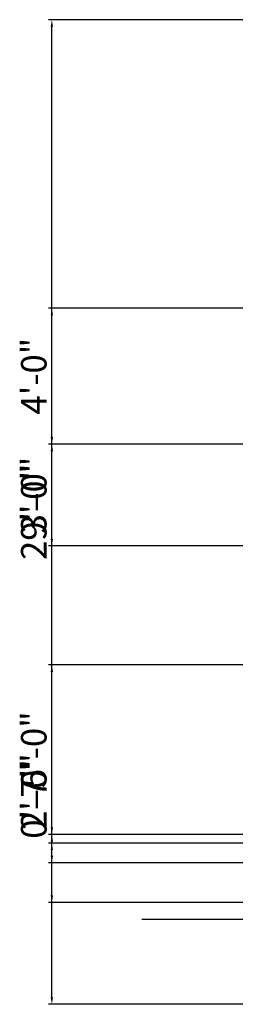
# Model space of a CAD drawing. Units: inches. Extents: x 600 to 1805, y 898 to 2057.
# Tile 1 of 5: x 1096 to 1172, y 938 to 1286. Entities that reach past the tile are written whole.
import ezdxf

# ---------------------------------------------------------------- set-up
doc = ezdxf.new("R2010")
doc.units = ezdxf.units.IN
doc.layers.add('A-ANNO-DIMS', color=2, linetype='Continuous', lineweight=18)
doc.layers.add('C-SITE', color=7, linetype='Continuous', lineweight=25)
doc.styles.get("Standard").update_dxf_attribs({"font": 'arial.ttf'})
doc.dimstyles.new('ISO-25', dxfattribs={"dimtxt": 9, "dimasz": 2.5, "dimexe": 1.25, "dimexo": 0.625, "dimtad": 1, "dimlunit": 3, "dimtxsty": 'Standard', "dimcen": 2.5, "dimadec": 0, "dimazin": 0, "dimtfac": 1, "dimtmove": 0, "dimatfit": 3, "dimfxl": 1, "dimarcsym": 0})

# ---------------------------------------------------------------- blocks, each defined once
blk = doc.blocks.new('*D42')
at = {"layer": 'A-ANNO-DIMS', "color": 0, "lineweight": -2, "transparency": 16777216}
for p, q in [((1406.71, 1285.8), (1106.33, 1285.8)), ((1107.58, 940.3), (1107.58, 1283.3)), ((1183.78, 937.8), (1106.33, 937.8))]:
    blk.add_line(p, q, dxfattribs=at)
at = {"layer": 'A-ANNO-DIMS', "color": 0, "transparency": 16777216}
for points in [[(1107.16, 1283.3), (1107.99, 1283.3), (1107.58, 1285.8)], [(1107.16, 940.3), (1107.99, 940.3), (1107.58, 937.8)]]:
    blk.add_solid(points, dxfattribs=at)
at = {"layer": 'Defpoints', "color": 0, "transparency": 16777216}
for p in [(1107.58, 1285.8), (1407.34, 1285.8), (1184.4, 937.8)]:
    blk.add_point(p, dxfattribs=at)
at = {"layer": 'A-ANNO-DIMS', "color": 0, "transparency": 16777216, "insert": (1102.36, 1111.8), "char_height": 9, "attachment_point": 5, "rotation": 90}
blk.add_mtext('29\'-0"', dxfattribs=at)
blk = doc.blocks.new('*D47')
at = {"layer": 'A-ANNO-DIMS', "color": 0, "lineweight": -2, "transparency": 16777216}
for p, q in [((1107.58, 994.8), (1107.58, 1022.48)), ((1562.71, 994.8), (1106.33, 994.8)), ((1107.58, 990.3), (1107.58, 992.3)), ((1562.71, 987.8), (1106.33, 987.8))]:
    blk.add_line(p, q, dxfattribs=at)
at = {"layer": 'A-ANNO-DIMS', "color": 0, "transparency": 16777216}
for points in [[(1107.16, 992.3), (1107.99, 992.3), (1107.58, 994.8)], [(1107.16, 990.3), (1107.99, 990.3), (1107.58, 987.8)]]:
    blk.add_solid(points, dxfattribs=at)
at = {"layer": 'Defpoints', "color": 0, "transparency": 16777216}
for p in [(1107.58, 994.8), (1563.34, 994.8), (1563.34, 987.8)]:
    blk.add_point(p, dxfattribs=at)
at = {"layer": 'A-ANNO-DIMS', "color": 0, "transparency": 16777216, "insert": (1102.36, 1009.89), "char_height": 9, "attachment_point": 5, "rotation": 90}
blk.add_mtext('0\'-7"', dxfattribs=at)
blk = doc.blocks.new('*D50')
at = {"layer": 'A-ANNO-DIMS', "color": 0, "lineweight": -2, "transparency": 16777216}
for p, q in [((1107.58, 997.8), (1107.58, 1025.63)), ((1208.71, 997.8), (1106.33, 997.8)), ((1107.58, 976.3), (1107.58, 995.3)), ((1208.71, 973.8), (1106.33, 973.8))]:
    blk.add_line(p, q, dxfattribs=at)
at = {"layer": 'A-ANNO-DIMS', "color": 0, "transparency": 16777216}
for points in [[(1107.16, 995.3), (1107.99, 995.3), (1107.58, 997.8)], [(1107.16, 976.3), (1107.99, 976.3), (1107.58, 973.8)]]:
    blk.add_solid(points, dxfattribs=at)
at = {"layer": 'Defpoints', "color": 0, "transparency": 16777216}
for p in [(1107.58, 997.8), (1209.34, 997.8), (1209.34, 973.8)]:
    blk.add_point(p, dxfattribs=at)
at = {"layer": 'A-ANNO-DIMS', "color": 0, "transparency": 16777216, "insert": (1102.36, 1012.97), "char_height": 9, "attachment_point": 5, "rotation": 90}
blk.add_mtext('2\'-0"', dxfattribs=at)
blk = doc.blocks.new('*D51')
at = {"layer": 'A-ANNO-DIMS', "color": 0, "lineweight": -2, "transparency": 16777216}
for p, q in [((1208.71, 1057.8), (1106.33, 1057.8)), ((1107.58, 1000.3), (1107.58, 1055.3)), ((1208.71, 997.8), (1106.33, 997.8))]:
    blk.add_line(p, q, dxfattribs=at)
at = {"layer": 'A-ANNO-DIMS', "color": 0, "transparency": 16777216}
for points in [[(1107.16, 1055.3), (1107.99, 1055.3), (1107.58, 1057.8)], [(1107.16, 1000.3), (1107.99, 1000.3), (1107.58, 997.8)]]:
    blk.add_solid(points, dxfattribs=at)
at = {"layer": 'Defpoints', "color": 0, "transparency": 16777216}
for p in [(1107.58, 1057.8), (1209.34, 1057.8), (1209.34, 997.8)]:
    blk.add_point(p, dxfattribs=at)
at = {"layer": 'A-ANNO-DIMS', "color": 0, "transparency": 16777216, "insert": (1102.36, 1027.8), "char_height": 9, "attachment_point": 5, "rotation": 90}
blk.add_mtext('5\'-0"', dxfattribs=at)
blk = doc.blocks.new('*D52')
at = {"layer": 'A-ANNO-DIMS', "color": 0, "lineweight": -2, "transparency": 16777216}
for p, q in [((1208.71, 1135.8), (1106.33, 1135.8)), ((1107.58, 1102.3), (1107.58, 1133.3)), ((1208.71, 1099.8), (1106.33, 1099.8))]:
    blk.add_line(p, q, dxfattribs=at)
at = {"layer": 'A-ANNO-DIMS', "color": 0, "transparency": 16777216}
for points in [[(1107.16, 1133.3), (1107.99, 1133.3), (1107.58, 1135.8)], [(1107.16, 1102.3), (1107.99, 1102.3), (1107.58, 1099.8)]]:
    blk.add_solid(points, dxfattribs=at)
at = {"layer": 'Defpoints', "color": 0, "transparency": 16777216}
for p in [(1107.58, 1135.8), (1209.34, 1135.8), (1209.34, 1099.8)]:
    blk.add_point(p, dxfattribs=at)
at = {"layer": 'A-ANNO-DIMS', "color": 0, "transparency": 16777216, "insert": (1102.35, 1117.8), "char_height": 9, "attachment_point": 5, "rotation": 90}
blk.add_mtext('3\'-0"', dxfattribs=at)
blk = doc.blocks.new('*D53')
at = {"layer": 'A-ANNO-DIMS', "color": 0, "lineweight": -2, "transparency": 16777216}
for p, q in [((1208.71, 1183.8), (1106.33, 1183.8)), ((1107.58, 1138.3), (1107.58, 1181.3)), ((1208.71, 1135.8), (1106.33, 1135.8))]:
    blk.add_line(p, q, dxfattribs=at)
at = {"layer": 'A-ANNO-DIMS', "color": 0, "transparency": 16777216}
for points in [[(1107.16, 1181.3), (1107.99, 1181.3), (1107.58, 1183.8)], [(1107.16, 1138.3), (1107.99, 1138.3), (1107.58, 1135.8)]]:
    blk.add_solid(points, dxfattribs=at)
at = {"layer": 'Defpoints', "color": 0, "transparency": 16777216}
for p in [(1107.58, 1183.8), (1209.34, 1183.8), (1209.34, 1135.8)]:
    blk.add_point(p, dxfattribs=at)
at = {"layer": 'A-ANNO-DIMS', "color": 0, "transparency": 16777216, "insert": (1102.36, 1159.8), "char_height": 9, "attachment_point": 5, "rotation": 90}
blk.add_mtext('4\'-0"', dxfattribs=at)

msp = doc.modelspace()

# ---------------------------------------------------------------- linework, layer by layer
at = {"layer": 'C-SITE'}
msp.add_line((1209.337, 967.803), (1139.301, 967.803), dxfattribs=at)

# ---------------------------------------------------------------- dimensions: what is measured, and where the dimension line sits
at = {"layer": 'A-ANNO-DIMS'}
for base, p1, p2, picture, middle in [((1107.576, 1285.803), (1184.402, 937.803), (1407.337, 1285.803), '*D42', (1102.356, 1111.803)), ((1107.576, 1183.803), (1209.337, 1135.803), (1209.337, 1183.803), '*D53', (1102.356, 1159.803)), ((1107.576, 1135.803), (1209.337, 1099.803), (1209.337, 1135.803), '*D52', (1102.353, 1117.803)), ((1107.576, 1057.803), (1209.337, 997.803), (1209.337, 1057.803), '*D51', (1102.356, 1027.803)), ((1107.576, 997.803), (1209.337, 973.803), (1209.337, 997.803), '*D50', (1102.356, 1012.967)), ((1107.576, 994.803), (1563.337, 987.803), (1563.337, 994.803), '*D47', (1102.356, 1009.89))]:
    dim = msp.add_linear_dim(base=base, p1=p1, p2=p2, angle=90, dimstyle='ISO-25', override={"dimdec": 1, "dimlfac": 1, "dimrnd": 0, "dimzin": 1, "dimdsep": 46, "dimlunit": 4, "dimfrac": 2}, dxfattribs=at)
    dim.commit()
    dim.dimension.update_dxf_attribs({"geometry": picture, "text_midpoint": middle})

doc.saveas('drawing.dxf')
